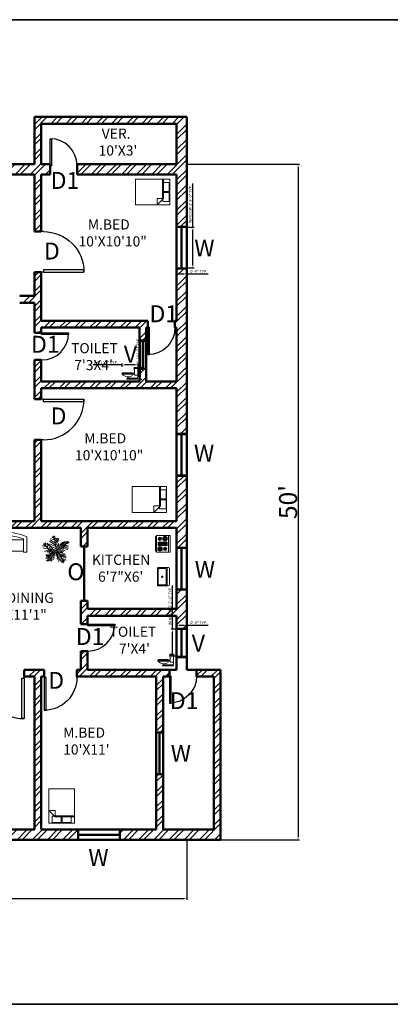
# Model space of a CAD drawing. Units: inches. Extents: x -31842 to -29388, y 18869 to 19743.
# Tile 4 of 12: x -31268 to -30939, y 18869 to 19743. Entities that reach past the tile are written whole.
import ezdxf

# ---------------------------------------------------------------- set-up
doc = ezdxf.new("R2010")
doc.units = ezdxf.units.IN
for name, color, linetype, lineweight in [('A-ANNO-DIMS', 2, 'Continuous', 18), ('A-ANNO-SYMB', 2, 'Continuous', 18), ('A-ANNO-TTLB', 7, 'Continuous', 35), ('A-AREA-IDEN', 3, 'Continuous', 18), ('A-DOOR', 3, 'Continuous', 25), ('A-FLOR-FIXT', 8, 'Continuous', 18), ('A-FURN', 8, 'Continuous', 18), ('A-GLAZ', 4, 'Continuous', 25), ('A-WALL', 7, 'Continuous', 50), ('A-WALL-PATT', 8, 'Continuous', 13), ('L-PLNT', 3, 'Continuous', 13)]:
    doc.layers.add(name, color=color, linetype=linetype, lineweight=lineweight)
doc.styles.get("Standard").update_dxf_attribs({"font": 'arial.ttf'})
doc.dimstyles.new('ISO-25', dxfattribs={"dimtxt": 2.5, "dimasz": 2.5, "dimexe": 1.25, "dimexo": 0.625, "dimtad": 1, "dimdec": 0, "dimlunit": 3, "dimtxsty": 'Standard', "dimcen": 2.5, "dimadec": 0, "dimazin": 0, "dimtfac": 1, "dimtdec": 0, "dimtmove": 0, "dimatfit": 3, "dimfxl": 1, "dimarcsym": 0})

# ---------------------------------------------------------------- blocks, each defined once
blk = doc.blocks.new('*U8')
for p, q in [((0, 0), (0, -100)), ((750, 0), (750, -100))]:
    blk.add_line(p, q)
blk.add_lwpolyline([(0, 0), (0, 750), (43.75, 750), (43.75, 0)], close=True)
blk.add_arc((0, 0), 750, 0, 90)
blk = doc.blocks.new('Bed - Queen')
for p, q in [((0, -80.00003), (0, 0)), ((0, 0), (59.99999, 0)), ((59.99999, 0), (59.99999, -80.00003)), ((0, -14.4), (44.8, -14.4)), ((44.8, -16.8), (0, -16.8)), ((7.99999, -1.2), (28.79998, -1.2)), ((7.99999, -14.4), (7.99999, -1.2)), ((28.79998, -1.2), (28.79998, -14.4)), ((31.19999, -1.2), (51.99999, -1.2)), ((31.19999, -14.4), (31.19999, -1.2)), ((59.99999, -29.6), (44.8, -14.4)), ((44.8, -14.4), (44.8, -29.6)), ((51.99999, -16.4), (46.79936, -16.4)), ((51.99999, -1.2), (51.99999, -16.4)), ((44.8, -29.6), (59.99999, -29.6)), ((59.99999, -80.00003), (0, -80.00003))]:
    blk.add_line(p, q)
blk = doc.blocks.new('Toilet - side')
for p, q in [((0.5, 5), (0.5, 22)), ((7.5, 22), (7.5, 12)), ((7.5, 21), (9, 21)), ((9, 21), (9, 20)), ((6, 8), (0.5, 8)), ((22, 2), (2, 2)), ((2, 2), (2, 1)), ((8, 10), (6, 8)), ((9, 20), (7.5, 20)), ((7.5, 12), (33, 12)), ((33, 10), (8, 10)), ((32.5, 13), (12, 13)), ((12, 13), (12, 12)), ((21, 4.5), (21, 2)), ((22, 2), (22, 4.5)), ((22, 1), (22, 2)), ((32.5, 12), (32.5, 13)), ((33, 12), (33, 10))]:
    blk.add_line(p, q)
for points in [[(0, 22), (0, 24), (8, 24), (8, 22)], [(1, 0), (1, 1), (23, 1), (23, 0)]]:
    blk.add_lwpolyline(points, close=True)
for centre, radius, start, end in [((3.8, 4.8), 3.26, 175.6013, 237.5288), ((20.3, 20.7), 16.2, 238.1872, 318.7702)]:
    blk.add_arc(centre, radius, start, end)
blk = doc.blocks.new('Range-Oven - 30 in top')
for p, q in [((0, -3), (30, -3)), ((12, -6), (18, -6)), ((13, -20), (13, -6)), ((14, -6), (14, -20)), ((15, -20), (15, -6)), ((16, -6), (16, -20)), ((17, -20), (17, -6)), ((6, -24), (6, -25)), ((8, -25), (8, -24)), ((18, -20), (12, -20)), ((22, -25), (22, -24)), ((24, -24), (24, -25))]:
    blk.add_line(p, q)
for points in [[(0, -24), (0, 0), (30, 0), (30, -24)], [(12, -21), (12, -5), (18, -5), (18, -21)], [(2, -26), (2, -25), (28, -25), (28, -26)]]:
    blk.add_lwpolyline(points, close=True)
for centre, radius in [((6, -9), 4), ((6, -9), 3), ((6, -18), 3), ((6, -9), 2), ((6, -18), 2), ((6, -9), 1), ((6, -18), 1), ((24, -18), 4), ((24, -9), 3), ((24, -18), 3), ((24, -9), 2), ((24, -18), 2), ((24, -9), 1), ((24, -18), 1)]:
    blk.add_circle(centre, radius)
blk = doc.blocks.new('Sink-single - 30 in top')
blk.add_line((-15, -3.999996), (15, -3.999996))
for points in [[(-13.5, 0), (13.5, 0)], [(-15, -18.499996), (-15, -1.5)], [(-13.5, -17.499996), (-13.5, -6.499996)], [(-12.5, -5.499996), (12.5, -5.499996)], [(13.5, -6.499996), (13.5, -17.499996)], [(15, -1.5), (15, -18.499996)], [(13.5, -19.999996), (-13.5, -19.999996)], [(12.5, -18.499996), (-12.5, -18.499996)]]:
    blk.add_lwpolyline(points)
for radius in [1, 0.5]:
    blk.add_circle((0, -11.999996), radius)
for centre, radius, start, end in [((-13.5, -1.5), 1.5, 90, 180), ((-12.5, -6.499996), 1, 90, 180), ((12.5, -6.499996), 1, 0, 90), ((13.5, -1.5), 1.5, 0, 90), ((-13.5, -18.499996), 1.5, 180, 270), ((-12.5, -17.499996), 1, 180, 270), ((12.5, -17.499996), 1, 270, 0), ((13.5, -18.499996), 1.5, 270, 0)]:
    blk.add_arc(centre, radius, start, end)
blk = doc.blocks.new('Sofa - Roundback 7 ft.')
for p, q in [((-36.000027, -34), (-36.000027, -11.4696)), ((-35.999844, -13.3819), (35.9998, -13.3819)), ((-12.00002, -32.4421), (-12.00003, -6.5971)), ((11.99997, -32.4421), (11.99998, -6.5971)), ((35.99998, -34), (35.99998, -11.4696)), ((-36.000027, -32.4421), (35.99998, -32.4421))]:
    blk.add_line(p, q)
for points in [[(-36.000027, -34), (-42.000027, -34), (-42.000027, -8)], [(41.99998, -8), (41.99998, -34), (35.99998, -34)]]:
    blk.add_lwpolyline(points)
for centre, radius, start, end in [((0, -114.25), 114.25, 68.43141, 111.5686), ((-0.00001, -127.1968), 121.1968, 72.72033, 107.2797)]:
    blk.add_arc(centre, radius, start, end)
blk = doc.blocks.new('*U122')
for p, q in [((-129.8956, 713.6638), (-626.7704, 1032.1544)), ((-185.1152, 1008.5578), (-553.1612, 1185.4942)), ((-221.9198, 1197.3052), (-433.5526, 1338.8594)), ((-258.7244, 1362.456), (-332.3336, 1421.4348)), ((0, 0), (-266.7, 1447.8)), ((-231.1146, 1315.2628), (-166.7002, 1421.4348)), ((-194.31, 1102.9442), (-65.4812, 1256.284)), ((-148.3106, 914.1968), (118.5418, 1220.9018)), ((-129.8956, 701.8528), (265.7602, 1185.4942)), ((-1206.4492, 501.3198), (-1418.082, 465.9376)), ((-1031.621, 347.98), (-1399.667, 277.1902)), ((-800.1, 114.3), (-1333.5, 647.7)), ((-847.598, 159.2326), (-1326.0578, 135.636)), ((-1234.059, 536.7274), (-1252.4486, 737.2604)), ((-718.7946, 88.4682), (-1215.644, -147.447)), ((-1105.2302, 725.4494), (-1077.6458, 395.1732)), ((-976.4268, 666.4706), (-884.4026, 194.6402)), ((-543.9664, 76.6572), (-967.2066, -206.4512)), ((-902.8176, 713.6638), (-617.5756, 100.2538)), ((0, 0), (-800.1, 114.3)), ((-369.1382, 53.086), (-783.1836, 642.874)), ((-405.9428, 53.086), (-764.794, -241.8334)), ((-93.091, 489.5342), (-700.3796, 902.3858)), ((-617.5756, 607.4918), (-74.7014, 347.98)), ((0, 0), (-571.5, -495.3)), ((-166.7002, 29.4894), (-543.9664, -206.4512)), ((-525.5514, 347.98), (-28.6766, 123.8504)), ((-74.7014, 418.7444), (219.7608, 961.39)), ((-28.6766, 171.0436), (228.9556, 678.2816)), ((0, 0), (685.8, 228.6)), ((0, 0), (457.2, -571.5)), ((100.1268, 41.275), (284.1498, 619.2774)), ((164.5412, 41.275), (661.416, -218.2368)), ((256.5654, 88.4682), (449.7832, 666.4706)), ((284.1498, 88.4682), (781.0246, -147.447)), ((412.9786, 147.447), (587.8068, 796.2392)), ((458.978, 147.447), (891.4384, -88.4682)), ((560.197, 182.8292), (698.2206, 819.8358)), ((615.4166, 194.6402), (1185.8752, 41.275)), ((685.8, 228.6), (1219.2, 914.4)), ((689.0258, 230.0224), (790.2448, 914.1968)), ((753.4148, 312.5978), (1222.6798, 159.2326)), ((808.6344, 784.4282), (827.0494, 418.7444)), ((845.439, 418.7444), (1241.0948, 277.1902)), ((891.4384, 831.6214), (946.658, 572.1096)), ((919.0482, 501.3198), (1222.6798, 454.152)), ((983.4626, 867.0036), (1066.2666, 725.4494)), ((1029.462, 654.685), (1241.0948, 631.0884)), ((1112.2914, 760.8316), (1296.3144, 784.4282)), ((1121.4862, 925.9824), (1149.0706, 831.6214)), ((-442.7474, -383.3876), (-1086.8406, -477.7486)), ((-718.7946, -737.2604), (-1086.8406, -796.2392)), ((-617.5756, -548.5384), (-1077.6458, -560.324)), ((-783.1836, -867.029), (-1077.6458, -902.4112)), ((-875.2078, -1008.5832), (-1040.8412, -1079.3476)), ((-681.9646, -666.496), (-1022.4262, -654.685)), ((-571.5, -495.3), (-952.5, -1143)), ((-829.2084, -937.7934), (-810.7934, -1126.5408)), ((-387.5278, -324.4088), (-764.794, -324.4088)), ((-737.1842, -784.4536), (-709.5744, -1114.7298)), ((-635.9652, -607.5172), (-580.771, -1150.1374)), ((-525.5514, -465.963), (-451.9422, -1126.5408)), ((-166.7002, -147.447), (-507.1618, -253.619)), ((-433.5526, -383.3876), (-323.1134, -1020.3688)), ((-341.5284, -289.0012), (-221.9198, -831.6214)), ((-240.3094, -218.2368), (-157.5054, -595.7062)), ((-120.7008, -88.4682), (-93.091, -371.5766)), ((63.3222, -76.6826), (-37.8714, -513.1308)), ((44.9326, -64.897), (615.4166, -241.8334)), ((127.7366, -159.258), (54.1274, -654.685)), ((228.9556, -289.0012), (90.932, -914.1968)), ((357.759, -430.5554), (164.5412, -1020.3688)), ((192.151, -230.0224), (817.8292, -371.5766)), ((458.978, -572.1096), (210.5406, -1161.923)), ((311.7596, -383.3876), (937.4378, -477.7486)), ((514.1976, -772.6426), (403.7838, -1138.3264)), ((412.9786, -501.3452), (919.0482, -583.9206)), ((457.2, -571.5), (685.8, -1333.5)), ((468.1982, -572.1096), (1029.462, -737.2604)), ((486.5878, -642.8994), (983.4626, -843.4324)), ((578.612, -961.39), (495.7826, -1232.7128)), ((541.8074, -831.6214), (992.6574, -1032.1544)), ((578.612, -973.1756), (873.0488, -1138.3264)), ((624.6114, -1161.923), (587.8068, -1291.6916)), ((624.6114, -1102.9442), (781.0246, -1209.1162)), ((679.8056, -1268.095), (716.6102, -1291.6916))]:
    blk.add_line(p, q)
blk = doc.blocks.new('*D197')
at = {"layer": 'A-ANNO-DIMS', "color": 0, "lineweight": -2, "transparency": 16777216}
for p, q in [((-31651.45, 19014.34), (-31651.45, 18961.52)), ((-31119.45, 19014.34), (-31119.45, 18961.52)), ((-31648.95, 18962.77), (-31121.95, 18962.77))]:
    blk.add_line(p, q, dxfattribs=at)
at = {"layer": 'A-ANNO-DIMS', "color": 0, "transparency": 16777216}
for points in [[(-31648.95, 18963.19), (-31648.95, 18962.35), (-31651.45, 18962.77)], [(-31121.95, 18963.19), (-31121.95, 18962.35), (-31119.45, 18962.77)]]:
    blk.add_solid(points, dxfattribs=at)
at = {"layer": 'Defpoints', "color": 0, "transparency": 16777216}
for p in [(-31651.45, 19014.96), (-31119.45, 19014.96), (-31119.45, 18962.77)]:
    blk.add_point(p, dxfattribs=at)
at = {"layer": 'A-ANNO-DIMS', "color": 0, "transparency": 16777216, "insert": (-31385.45, 18971.4), "char_height": 2.5, "attachment_point": 5}
blk.add_mtext('{\\H6.4x;44\'-4"}', dxfattribs=at)
blk = doc.blocks.new('*D198')
at = {"layer": 'A-ANNO-DIMS', "color": 0, "lineweight": -2, "transparency": 16777216}
for p, q in [((-31118.83, 19614.96), (-31019.53, 19614.96)), ((-31020.78, 19612.46), (-31020.78, 19017.46)), ((-31118.83, 19014.96), (-31019.53, 19014.96))]:
    blk.add_line(p, q, dxfattribs=at)
at = {"layer": 'A-ANNO-DIMS', "color": 0, "transparency": 16777216}
for points in [[(-31021.19, 19612.46), (-31020.36, 19612.46), (-31020.78, 19614.96)], [(-31021.19, 19017.46), (-31020.36, 19017.46), (-31020.78, 19014.96)]]:
    blk.add_solid(points, dxfattribs=at)
at = {"layer": 'Defpoints', "color": 0, "transparency": 16777216}
for p in [(-31119.45, 19614.96), (-31119.45, 19014.96), (-31020.78, 19014.96)]:
    blk.add_point(p, dxfattribs=at)
at = {"layer": 'A-ANNO-DIMS', "color": 0, "transparency": 16777216, "insert": (-31029.57, 19314.96), "char_height": 2.5, "attachment_point": 5, "rotation": 90}
blk.add_mtext("{\\H6.4x;50'}", dxfattribs=at)
blk = doc.blocks.new('WIN-3FT')
for p, q in [((0, 36), (9, 36)), ((4, 0), (4, 36)), ((4.5, 0), (4.5, 36)), ((5, 0), (5, 36)), ((0, 0), (9, 0))]:
    blk.add_line(p, q)
blk = doc.blocks.new('WIN-3FT-B')
for p, q in [((0, 36), (6, 36)), ((2.5, 0), (2.5, 36)), ((3, 0), (3, 36)), ((3.5, 0), (3.5, 36)), ((0, 0), (6, 0))]:
    blk.add_line(p, q)
blk = doc.blocks.new('WIN-2FT')
for p, q in [((0, 24), (9, 24)), ((4, 0), (4, 24)), ((4.5, 0), (4.5, 24)), ((5, 0), (5, 24)), ((0, 0), (9, 0))]:
    blk.add_line(p, q)
blk = doc.blocks.new('*D217')
at = {"layer": 'A-ANNO-DIMS', "color": 0, "lineweight": -2, "transparency": 16777216}
for p, q in [((-31114.05, 19558.96), (-31114.05, 19597.93)), ((-31118.83, 19558.96), (-31112.8, 19558.96)), ((-31114.05, 19525.46), (-31114.05, 19556.46)), ((-31118.83, 19522.96), (-31112.8, 19522.96))]:
    blk.add_line(p, q, dxfattribs=at)
at = {"layer": 'A-ANNO-DIMS', "color": 0, "transparency": 16777216}
for points in [[(-31114.47, 19556.46), (-31113.64, 19556.46), (-31114.05, 19558.96)], [(-31114.47, 19525.46), (-31113.64, 19525.46), (-31114.05, 19522.96)]]:
    blk.add_solid(points, dxfattribs=at)
at = {"layer": 'Defpoints', "color": 0, "transparency": 16777216}
for p in [(-31119.45, 19558.96), (-31114.05, 19558.96), (-31119.45, 19522.96)]:
    blk.add_point(p, dxfattribs=at)
at = {"layer": 'A-ANNO-DIMS', "color": 0, "transparency": 16777216, "insert": (-31115.97, 19579.69), "char_height": 2.5, "attachment_point": 5, "rotation": 90}
blk.add_mtext('WINDOW 3\' 3\'-0" TYP.', dxfattribs=at)
blk = doc.blocks.new('*D218')
at = {"layer": 'A-ANNO-DIMS', "color": 0, "lineweight": -2, "transparency": 16777216}
for p, q in [((-31128.45, 19522.34), (-31128.45, 19516.31)), ((-31119.45, 19522.34), (-31119.45, 19516.31)), ((-31125.95, 19517.56), (-31121.95, 19517.56)), ((-31119.45, 19517.56), (-31100.46, 19517.56))]:
    blk.add_line(p, q, dxfattribs=at)
at = {"layer": 'A-ANNO-DIMS', "color": 0, "transparency": 16777216}
for points in [[(-31125.95, 19517.98), (-31125.95, 19517.14), (-31128.45, 19517.56)], [(-31121.95, 19517.98), (-31121.95, 19517.14), (-31119.45, 19517.56)]]:
    blk.add_solid(points, dxfattribs=at)
at = {"layer": 'Defpoints', "color": 0, "transparency": 16777216}
for p in [(-31128.45, 19522.96), (-31119.45, 19522.96), (-31119.45, 19517.56)]:
    blk.add_point(p, dxfattribs=at)
at = {"layer": 'A-ANNO-DIMS', "color": 0, "transparency": 16777216, "insert": (-31108.71, 19519.46), "char_height": 2.5, "attachment_point": 5}
blk.add_mtext('0\'-9" TYP.', dxfattribs=at)
blk = doc.blocks.new('*D225')
at = {"layer": 'A-ANNO-DIMS', "color": 0, "lineweight": -2, "transparency": 16777216}
for p, q in [((-31176.87, 19436.68), (-31202.75, 19436.68)), ((-31176.87, 19435.17), (-31176.87, 19437.93)), ((-31165.13, 19436.68), (-31174.37, 19436.68)), ((-31162.63, 19435.17), (-31162.63, 19437.93))]:
    blk.add_line(p, q, dxfattribs=at)
at = {"layer": 'A-ANNO-DIMS', "color": 0, "transparency": 16777216}
for points in [[(-31174.37, 19437.09), (-31174.37, 19436.26), (-31176.87, 19436.68)], [(-31165.13, 19437.09), (-31165.13, 19436.26), (-31162.63, 19436.68)]]:
    blk.add_solid(points, dxfattribs=at)
at = {"layer": 'Defpoints', "color": 0, "transparency": 16777216}
for p in [(-31176.87, 19436.68), (-31176.87, 19434.54), (-31162.63, 19434.54)]:
    blk.add_point(p, dxfattribs=at)
at = {"layer": 'A-ANNO-DIMS', "color": 0, "transparency": 16777216, "insert": (-31191.06, 19438.59), "char_height": 2.5, "attachment_point": 5}
blk.add_mtext('WC 1\'-2" TYP.', dxfattribs=at)
blk = doc.blocks.new('*D226')
at = {"layer": 'A-ANNO-DIMS', "color": 0, "lineweight": -2, "transparency": 16777216}
for p, q in [((-31160.49, 19434.54), (-31160.49, 19461.3)), ((-31162.01, 19434.54), (-31159.24, 19434.54)), ((-31162.01, 19424.19), (-31159.24, 19424.19)), ((-31160.49, 19426.69), (-31160.49, 19432.04))]:
    blk.add_line(p, q, dxfattribs=at)
at = {"layer": 'A-ANNO-DIMS', "color": 0, "transparency": 16777216}
for points in [[(-31160.91, 19432.04), (-31160.08, 19432.04), (-31160.49, 19434.54)], [(-31160.91, 19426.69), (-31160.08, 19426.69), (-31160.49, 19424.19)]]:
    blk.add_solid(points, dxfattribs=at)
at = {"layer": 'Defpoints', "color": 0, "transparency": 16777216}
for p in [(-31162.63, 19434.54), (-31160.49, 19434.54), (-31162.63, 19424.19)]:
    blk.add_point(p, dxfattribs=at)
at = {"layer": 'A-ANNO-DIMS', "color": 0, "transparency": 16777216, "insert": (-31162.41, 19449.17), "char_height": 2.5, "attachment_point": 5, "rotation": 90}
blk.add_mtext('0\'-10 1/2" TYP.', dxfattribs=at)
blk = doc.blocks.new('*D259')
at = {"layer": 'A-ANNO-DIMS', "color": 0, "lineweight": -2, "transparency": 16777216}
for p, q in [((-31132.05, 19201.96), (-31132.05, 19240.93)), ((-31129.08, 19201.96), (-31133.3, 19201.96)), ((-31132.05, 19180.46), (-31132.05, 19199.46)), ((-31129.08, 19177.96), (-31133.3, 19177.96))]:
    blk.add_line(p, q, dxfattribs=at)
at = {"layer": 'A-ANNO-DIMS', "color": 0, "transparency": 16777216}
for points in [[(-31132.47, 19199.46), (-31131.64, 19199.46), (-31132.05, 19201.96)], [(-31132.47, 19180.46), (-31131.64, 19180.46), (-31132.05, 19177.96)]]:
    blk.add_solid(points, dxfattribs=at)
at = {"layer": 'Defpoints', "color": 0, "transparency": 16777216}
for p in [(-31132.05, 19201.96), (-31128.45, 19201.96), (-31128.45, 19177.96)]:
    blk.add_point(p, dxfattribs=at)
at = {"layer": 'A-ANNO-DIMS', "color": 0, "transparency": 16777216, "insert": (-31133.97, 19222.69), "char_height": 2.5, "attachment_point": 5, "rotation": 90}
blk.add_mtext('WINDOW 2\' 2\'-0" TYP.', dxfattribs=at)
blk = doc.blocks.new('*D260')
at = {"layer": 'A-ANNO-DIMS', "color": 0, "lineweight": -2, "transparency": 16777216}
for p, q in [((-31128.45, 19202.59), (-31128.45, 19206.81)), ((-31125.95, 19205.56), (-31121.95, 19205.56)), ((-31119.45, 19202.59), (-31119.45, 19206.81)), ((-31119.45, 19205.56), (-31100.46, 19205.56))]:
    blk.add_line(p, q, dxfattribs=at)
at = {"layer": 'A-ANNO-DIMS', "color": 0, "transparency": 16777216}
for points in [[(-31125.95, 19205.98), (-31125.95, 19205.14), (-31128.45, 19205.56)], [(-31121.95, 19205.98), (-31121.95, 19205.14), (-31119.45, 19205.56)]]:
    blk.add_solid(points, dxfattribs=at)
at = {"layer": 'Defpoints', "color": 0, "transparency": 16777216}
for p in [(-31119.45, 19205.56), (-31128.45, 19201.96), (-31119.45, 19201.96)]:
    blk.add_point(p, dxfattribs=at)
at = {"layer": 'A-ANNO-DIMS', "color": 0, "transparency": 16777216, "insert": (-31108.71, 19207.46), "char_height": 2.5, "attachment_point": 5}
blk.add_mtext('0\'-9" TYP.', dxfattribs=at)

msp = doc.modelspace()

# ---------------------------------------------------------------- hatches: boundary and pattern name
at = {"layer": 'A-WALL-PATT'}
h = msp.add_hatch(dxfattribs=at)
h.set_pattern_fill('ANSI32', color=256)
h.paths.add_polyline_path([(-31119.45, 19656.96), (-31254.45, 19656.96), (-31254.45, 19614.96), (-31277.45, 19614.96), (-31277.45, 19605.96), (-31254.45, 19605.96), (-31254.45, 19555.2), (-31248.45, 19555.2), (-31248.45, 19605.96), (-31240.75, 19605.96), (-31240.75, 19614.96), (-31248.45, 19614.96), (-31248.45, 19650.96), (-31128.45, 19650.96), (-31128.45, 19614.96), (-31216.75, 19614.96), (-31216.75, 19605.96), (-31128.45, 19605.96), (-31128.45, 19559.96), (-31119.45, 19559.96)])
h.paths.add_polyline_path([(-31153.94, 19473.06), (-31153.92, 19475.96), (-31248.45, 19475.96), (-31248.45, 19519.2), (-31251.45, 19519.2), (-31254.45, 19519.2), (-31254.45, 19497.96), (-31267.62, 19497.96), (-31267.62, 19491.96), (-31254.45, 19491.96), (-31254.45, 19465.12), (-31248.45, 19465.12), (-31248.45, 19469.96), (-31161.45, 19469.96), (-31161.45, 19458.96), (-31155.45, 19458.96), (-31155.45, 19469.96), (-31153.94, 19469.96)])
h.paths.add_polyline_path([(-31119.45, 19521.96), (-31128.45, 19521.96), (-31128.45, 19475.96), (-31129.92, 19475.96), (-31129.92, 19469.96), (-31128.45, 19469.96), (-31128.45, 19421.96), (-31155.45, 19421.96), (-31155.45, 19432.96), (-31161.45, 19432.96), (-31161.45, 19421.96), (-31248.45, 19421.96), (-31248.45, 19441.12), (-31254.45, 19441.12), (-31254.45, 19406.17), (-31248.45, 19406.17), (-31248.45, 19415.96), (-31128.45, 19415.96), (-31128.45, 19375.96), (-31119.45, 19375.96)])
h.paths.add_polyline_path([(-31315.45, 19614.96), (-31366.45, 19614.96), (-31366.45, 19605.96), (-31344.45, 19605.96), (-31344.45, 19456.39), (-31338.45, 19456.39), (-31338.45, 19491.96), (-31328.43, 19491.96), (-31328.43, 19497.96), (-31338.45, 19497.96), (-31338.45, 19605.96), (-31315.45, 19605.96)])
h.paths.add_polyline_path([(-31404.45, 19614.96), (-31455.1, 19614.96), (-31455.1, 19605.96), (-31432.45, 19605.96), (-31432.45, 19497.96), (-31448.67, 19497.96), (-31448.67, 19491.96), (-31432.45, 19491.96), (-31432.45, 19456.39), (-31429.07, 19456.39), (-31426.45, 19456.39), (-31426.45, 19605.96), (-31404.45, 19605.96)])
h.paths.add_polyline_path([(-31493.1, 19614.96), (-31516.45, 19614.96), (-31516.45, 19656.96), (-31651.45, 19656.96), (-31651.45, 19559.96), (-31642.45, 19559.96), (-31642.45, 19605.96), (-31556.65, 19605.96), (-31556.65, 19614.96), (-31642.45, 19614.96), (-31642.45, 19650.96), (-31522.45, 19650.96), (-31522.45, 19614.96), (-31532.65, 19614.96), (-31532.65, 19613.66), (-31532.65, 19610.46), (-31532.65, 19605.96), (-31522.45, 19605.96), (-31522.45, 19541.95), (-31516.45, 19541.95), (-31516.45, 19605.96), (-31493.1, 19605.96)])
h.paths.add_polyline_path([(-31642.45, 19521.96), (-31651.45, 19521.96), (-31651.45, 19374.96), (-31642.45, 19374.96), (-31642.45, 19415.96), (-31522.45, 19415.96), (-31522.45, 19406.54), (-31516.45, 19406.54), (-31516.45, 19441.56), (-31522.45, 19441.56), (-31522.45, 19421.96), (-31609.45, 19421.96), (-31609.45, 19432.96), (-31615.45, 19432.96), (-31615.45, 19421.96), (-31642.45, 19421.96), (-31642.45, 19469.96), (-31641.6, 19469.96), (-31641.6, 19475.96), (-31642.45, 19475.96)])
h.paths.add_polyline_path([(-31516.45, 19491.96), (-31506.54, 19491.96), (-31506.54, 19497.96), (-31516.45, 19497.96), (-31516.45, 19505.95), (-31522.45, 19505.95), (-31522.45, 19475.96), (-31617.6, 19475.96), (-31617.6, 19469.96), (-31615.45, 19469.96), (-31615.45, 19458.96), (-31609.45, 19458.96), (-31609.45, 19469.96), (-31522.45, 19469.96), (-31522.45, 19465.56), (-31516.45, 19465.56)])
h.paths.add_polyline_path([(-31248.45, 19370.17), (-31251.45, 19370.17), (-31254.45, 19370.17), (-31254.45, 19297.96), (-31338.45, 19297.96), (-31338.45, 19420.39), (-31344.45, 19420.39), (-31344.45, 19413.96), (-31346.02, 19413.96), (-31346.02, 19407.96), (-31344.45, 19407.96), (-31344.45, 19291.96), (-31213.45, 19291.96), (-31213.45, 19275.43), (-31207.45, 19275.43), (-31207.45, 19291.96), (-31128.45, 19291.96), (-31128.45, 19274.96), (-31119.45, 19274.96), (-31119.45, 19337.96), (-31128.45, 19337.96), (-31128.45, 19297.96), (-31248.45, 19297.96)])
h.paths.add_polyline_path([(-31426.45, 19407.96), (-31424.99, 19407.96), (-31424.99, 19410.83), (-31424.95, 19413.96), (-31426.45, 19413.96), (-31426.45, 19420.39), (-31432.45, 19420.39), (-31432.45, 19295.96), (-31516.45, 19295.96), (-31516.45, 19370.54), (-31522.45, 19370.54), (-31522.45, 19295.96), (-31642.45, 19295.96), (-31642.45, 19336.96), (-31651.45, 19336.96), (-31651.45, 19272.96), (-31642.45, 19272.96), (-31642.45, 19289.96), (-31563.45, 19289.96), (-31563.45, 19270.05), (-31557.45, 19270.05), (-31557.45, 19289.96), (-31426.45, 19289.96)])
h.paths.add_polyline_path([(-31557.45, 19222.83), (-31563.45, 19222.83), (-31563.45, 19217.96), (-31642.45, 19217.96), (-31642.45, 19234.96), (-31651.45, 19234.96), (-31651.45, 19201.96), (-31642.45, 19201.96), (-31642.45, 19211.96), (-31563.45, 19211.96), (-31563.45, 19206.27), (-31562.72, 19206.27), (-31559.53, 19206.27), (-31557.45, 19206.18)])
h.paths.add_polyline_path([(-31553.97, 19163.65), (-31553.95, 19165.96), (-31557.45, 19165.96), (-31557.45, 19182.18), (-31563.45, 19182.18), (-31563.45, 19165.96), (-31639.16, 19165.96), (-31639.16, 19159.96), (-31630.45, 19159.96), (-31630.45, 19110.96), (-31624.45, 19110.96), (-31624.45, 19159.96), (-31553.97, 19159.96)])
h.paths.add_polyline_path([(-31663.16, 19165.96), (-31681.45, 19165.96), (-31681.45, 19014.96), (-31592.45, 19014.96), (-31592.45, 19023.96), (-31624.45, 19023.96), (-31624.45, 19072.96), (-31630.45, 19072.96), (-31630.45, 19023.96), (-31675.45, 19023.96), (-31675.45, 19159.96), (-31663.16, 19159.96)])
h.paths.add_polyline_path([(-31516.45, 19159.96), (-31505.99, 19159.96), (-31505.99, 19165.96), (-31524.95, 19165.96), (-31524.95, 19159.96), (-31522.45, 19159.96), (-31522.45, 19023.96), (-31554.45, 19023.96), (-31554.45, 19014.96), (-31471.45, 19014.96), (-31471.45, 19023.96), (-31516.45, 19023.96)])
h.paths.add_polyline_path([(-31337.45, 19023.96), (-31382.45, 19023.96), (-31382.45, 19159.96), (-31299.75, 19159.96), (-31299.75, 19165.96), (-31344.45, 19165.96), (-31382.45, 19165.96), (-31382.45, 19407.96), (-31382.02, 19413.96), (-31388.95, 19413.96), (-31388.95, 19407.96), (-31388.45, 19407.96), (-31388.45, 19165.96), (-31432.45, 19165.96), (-31469.99, 19165.96), (-31469.99, 19159.96), (-31432.45, 19159.96), (-31388.45, 19159.96), (-31388.45, 19023.96), (-31433.45, 19023.96), (-31433.45, 19014.96), (-31337.45, 19014.96)])
h.paths.add_polyline_path([(-31216.45, 19023.96), (-31248.45, 19023.96), (-31248.45, 19159.96), (-31245.93, 19159.96), (-31245.93, 19162.87), (-31245.93, 19165.96), (-31254.45, 19165.96), (-31263.75, 19165.96), (-31263.75, 19159.96), (-31254.45, 19159.96), (-31254.45, 19023.96), (-31299.45, 19023.96), (-31299.45, 19014.96), (-31216.45, 19014.96)])
h.paths.add_polyline_path([(-31089.45, 19165.96), (-31110.75, 19165.96), (-31110.75, 19159.96), (-31095.45, 19159.96), (-31095.45, 19023.96), (-31140.45, 19023.96), (-31140.45, 19072.96), (-31146.45, 19072.96), (-31146.45, 19023.96), (-31178.45, 19023.96), (-31178.45, 19014.96), (-31089.45, 19014.96)])
h.paths.add_polyline_path([(-31134.75, 19165.96), (-31207.45, 19165.96), (-31207.45, 19182.5), (-31213.45, 19182.5), (-31213.45, 19165.96), (-31216.93, 19165.96), (-31216.93, 19159.96), (-31146.45, 19159.96), (-31146.45, 19110.96), (-31140.45, 19110.96), (-31140.45, 19159.96), (-31134.75, 19159.96)])
h.paths.add_polyline_path([(-31119.45, 19236.96), (-31128.45, 19236.96), (-31128.45, 19219.96), (-31207.45, 19219.96), (-31207.45, 19227.12), (-31213.45, 19227.12), (-31213.45, 19206.5), (-31207.45, 19206.5), (-31207.45, 19213.96), (-31128.45, 19213.96), (-31128.45, 19202.96), (-31119.45, 19202.96)])

# ---------------------------------------------------------------- linework, layer by layer
at = {"layer": 'A-ANNO-TTLB'}
msp.add_lwpolyline([(-31842.18, 19743.36), (-29387.67, 19743.36), (-29387.67, 18868.82), (-31842.18, 18868.82)], close=True, dxfattribs=at)
at = {"layer": 'A-GLAZ'}
for p, q in [((-31128.45, 19559.96), (-31119.45, 19559.96)), ((-31128.45, 19521.96), (-31119.45, 19521.96)), ((-31161.45, 19458.96), (-31155.45, 19458.96)), ((-31161.45, 19458.96), (-31155.45, 19458.96)), ((-31161.45, 19457.96), (-31155.45, 19457.96)), ((-31161.45, 19457.96), (-31155.45, 19457.96)), ((-31158.95, 19457.96), (-31158.95, 19433.96)), ((-31158.95, 19457.96), (-31158.95, 19433.96)), ((-31158.45, 19457.96), (-31158.45, 19433.96)), ((-31158.45, 19457.96), (-31158.45, 19433.96)), ((-31157.95, 19457.96), (-31157.95, 19433.96)), ((-31157.95, 19457.96), (-31157.95, 19433.96)), ((-31161.45, 19433.96), (-31155.45, 19433.96)), ((-31161.45, 19433.96), (-31155.45, 19433.96)), ((-31161.45, 19432.96), (-31155.45, 19432.96)), ((-31161.45, 19432.96), (-31155.45, 19432.96)), ((-31128.45, 19375.96), (-31119.45, 19375.96)), ((-31128.45, 19337.96), (-31119.45, 19337.96)), ((-31128.45, 19274.96), (-31119.45, 19274.96)), ((-31128.45, 19236.96), (-31119.45, 19236.96)), ((-31128.45, 19202.96), (-31119.45, 19202.96)), ((-31128.45, 19176.96), (-31119.45, 19176.96)), ((-31146.45, 19110.96), (-31140.45, 19110.96)), ((-31146.45, 19072.96), (-31140.45, 19072.96)), ((-31216.45, 19023.96), (-31216.45, 19014.96)), ((-31178.45, 19023.96), (-31178.45, 19014.96))]:
    msp.add_line(p, q, dxfattribs=at)
at = {"layer": 'A-WALL'}
for p, q in [((-31254.45, 19656.96), (-31254.45, 19614.96)), ((-31254.45, 19656.96), (-31119.45, 19656.96)), ((-31248.45, 19650.96), (-31248.45, 19614.96)), ((-31248.45, 19650.96), (-31128.45, 19650.96)), ((-31128.45, 19650.96), (-31128.45, 19614.96)), ((-31119.45, 19656.96), (-31119.45, 19165.96)), ((-31516.45, 19614.96), (-31254.45, 19614.96)), ((-31248.45, 19614.96), (-31240.75, 19614.96)), ((-31240.75, 19614.96), (-31240.75, 19605.96)), ((-31216.75, 19614.96), (-31216.75, 19605.96)), ((-31216.75, 19614.96), (-31128.45, 19614.96)), ((-31338.45, 19605.96), (-31254.45, 19605.96)), ((-31254.45, 19605.96), (-31254.45, 19555.2)), ((-31248.45, 19605.96), (-31240.75, 19605.96)), ((-31248.45, 19605.96), (-31248.45, 19555.2)), ((-31216.75, 19605.96), (-31128.45, 19605.96)), ((-31128.45, 19605.96), (-31128.45, 19475.96)), ((-31254.45, 19555.2), (-31248.45, 19555.2)), ((-31254.45, 19519.2), (-31248.45, 19519.2)), ((-31254.45, 19519.2), (-31254.45, 19497.96)), ((-31248.45, 19519.2), (-31248.45, 19475.96)), ((-31267.62, 19497.96), (-31254.45, 19497.96)), ((-31267.62, 19491.96), (-31254.45, 19491.96)), ((-31254.45, 19491.96), (-31254.45, 19465.12)), ((-31248.45, 19475.96), (-31153.92, 19475.96)), ((-31153.92, 19475.96), (-31153.92, 19469.96)), ((-31129.92, 19475.96), (-31129.92, 19469.96)), ((-31129.92, 19475.96), (-31128.45, 19475.96)), ((-31248.45, 19469.96), (-31161.45, 19469.96)), ((-31248.45, 19469.96), (-31248.45, 19465.12)), ((-31161.45, 19469.96), (-31161.45, 19421.96)), ((-31155.45, 19469.96), (-31153.92, 19469.96)), ((-31155.45, 19469.96), (-31155.45, 19421.96)), ((-31129.92, 19469.96), (-31128.45, 19469.96)), ((-31128.45, 19469.96), (-31128.45, 19421.96)), ((-31254.45, 19465.12), (-31248.45, 19465.12)), ((-31254.45, 19441.12), (-31248.45, 19441.12)), ((-31254.45, 19441.12), (-31254.45, 19406.17)), ((-31248.45, 19441.12), (-31248.45, 19421.96)), ((-31248.45, 19421.96), (-31161.45, 19421.96)), ((-31248.45, 19415.96), (-31128.45, 19415.96)), ((-31248.45, 19415.96), (-31248.45, 19406.17)), ((-31155.45, 19421.96), (-31128.45, 19421.96)), ((-31128.45, 19415.96), (-31128.45, 19297.96)), ((-31254.45, 19406.17), (-31248.45, 19406.17)), ((-31254.45, 19370.17), (-31248.45, 19370.17)), ((-31254.45, 19370.17), (-31254.45, 19297.96)), ((-31248.45, 19370.17), (-31248.45, 19297.96)), ((-31338.45, 19297.96), (-31254.45, 19297.96)), ((-31248.45, 19297.96), (-31128.45, 19297.96)), ((-31344.45, 19291.96), (-31213.45, 19291.96)), ((-31213.45, 19291.96), (-31213.45, 19275.43)), ((-31207.45, 19291.96), (-31207.45, 19275.43)), ((-31207.45, 19291.96), (-31128.45, 19291.96)), ((-31128.45, 19291.96), (-31128.45, 19219.96)), ((-31213.45, 19275.43), (-31207.45, 19275.43)), ((-31210.45, 19227.12), (-31210.45, 19275.43)), ((-31213.45, 19227.12), (-31207.45, 19227.12)), ((-31213.45, 19227.12), (-31213.45, 19206.5)), ((-31207.45, 19227.12), (-31207.45, 19219.96)), ((-31207.45, 19219.96), (-31128.45, 19219.96)), ((-31207.45, 19213.96), (-31128.45, 19213.96)), ((-31207.45, 19213.96), (-31207.45, 19206.5)), ((-31128.45, 19213.96), (-31128.45, 19165.96)), ((-31213.45, 19206.5), (-31207.45, 19206.5)), ((-31213.45, 19182.5), (-31207.45, 19182.5)), ((-31213.45, 19182.5), (-31213.45, 19165.96)), ((-31207.45, 19182.5), (-31207.45, 19165.96)), ((-31263.75, 19159.96), (-31263.75, 19165.96)), ((-31263.75, 19165.96), (-31254.45, 19165.96)), ((-31254.45, 19165.96), (-31245.93, 19165.96)), ((-31245.93, 19159.96), (-31245.93, 19165.96)), ((-31216.93, 19159.96), (-31216.93, 19165.96)), ((-31216.93, 19165.96), (-31213.45, 19165.96)), ((-31207.45, 19165.96), (-31128.45, 19165.96)), ((-31134.75, 19165.96), (-31134.75, 19159.96)), ((-31119.45, 19165.96), (-31089.45, 19165.96)), ((-31110.75, 19165.96), (-31110.75, 19159.96)), ((-31089.45, 19165.96), (-31089.45, 19014.96)), ((-31263.75, 19159.96), (-31254.45, 19159.96)), ((-31254.45, 19159.96), (-31254.45, 19023.96)), ((-31248.45, 19159.96), (-31248.45, 19023.96)), ((-31248.45, 19159.96), (-31245.93, 19159.96)), ((-31216.93, 19159.96), (-31146.45, 19159.96)), ((-31146.45, 19159.96), (-31146.45, 19023.96)), ((-31140.45, 19159.96), (-31140.45, 19023.96)), ((-31140.45, 19159.96), (-31134.75, 19159.96)), ((-31110.75, 19159.96), (-31095.45, 19159.96)), ((-31095.45, 19159.96), (-31095.45, 19023.96)), ((-31254.45, 19023.96), (-31382.45, 19023.96)), ((-31146.45, 19023.96), (-31248.45, 19023.96)), ((-31095.45, 19023.96), (-31140.45, 19023.96)), ((-31089.45, 19014.96), (-31681.45, 19014.96))]:
    msp.add_line(p, q, dxfattribs=at)

# ---------------------------------------------------------------- block references
at = {"layer": 'A-DOOR', "xscale": 0.0320000000000009, "yscale": 0.0320000000000009, "zscale": 0.0320000000000009}
msp.add_blockref('*U8', (-31240.75, 19613.66), dxfattribs=at)
at = {"layer": 'A-DOOR'}
for p, xscale, yscale, zscale, rotation in [((-31246.65, 19519.2), -0.0480000009996888, 0.0480000009996888, 0.0480000009996888, 270), ((-31153.94, 19469.86), -0.03199974142424, 0.03199974142424, 0.03199974142424, 180), ((-31248.25, 19465.12), 0.0320000009996884, 0.0320000009996884, 0.0320000009996884, 270), ((-31246.65, 19406.17), 0.0479999979369979, 0.0479999979369979, 0.0479999979369979, 270), ((-31207.25, 19206.5), 0.0320000009996884, 0.0320000009996884, 0.0320000009996884, 270), ((-31263.75, 19158.56), 0.0480000000000001, 0.0480000000000001, 0.0480000000000001, 180), ((-31245.93, 19159), -0.0386670485405529, 0.0386670485405529, 0.0386670485405529, 180), ((-31134.76, 19160.28), -0.03199974142424, 0.03199974142424, 0.03199974142424, 180)]:
    msp.add_blockref('*U8', p, dxfattribs=dict(at, xscale=xscale, yscale=yscale, zscale=zscale, rotation=rotation))
at = {"layer": 'A-FLOR-FIXT', "xscale": -0.4314503559530352, "yscale": 0.4314503559530352, "zscale": 0.4314503559530352}
for p in [(-31162.63, 19424.19), (-31130.91, 19169.34)]:
    msp.add_blockref('Toilet - side', p, dxfattribs=at)
at = {"layer": 'A-FLOR-FIXT', "rotation": 270}
for name, p, xscale, yscale, zscale in [('Range-Oven - 30 in top', (-31134.22, 19285.35), 0.501109879279097, 0.501109879279097, 0.501109879279097), ('Sink-single - 30 in top', (-31134.75, 19248.59), 0.537483841617589, 0.537483841617589, 0.537483841617589)]:
    msp.add_blockref(name, p, dxfattribs=dict(at, xscale=xscale, yscale=yscale, zscale=zscale))
at = {"layer": 'A-FURN', "xscale": 0.382279819255463, "yscale": 0.382279819255463, "zscale": 0.382279819255463}
for p, rotation in [((-31134.48, 19601.79), 270), ((-31137.36, 19328.69), 270), ((-31218.92, 19029.74), 180)]:
    msp.add_blockref('Bed - Queen', p, dxfattribs=dict(at, rotation=rotation))
at = {"layer": 'A-FURN', "xscale": 0.5237896943857897, "yscale": 0.5237896943857897, "zscale": 0.5237896943857897}
msp.add_blockref('Sofa - Roundback 7 ft.', (-31283.23, 19288.36), dxfattribs=at)
at = {"layer": 'A-GLAZ'}
for name, p in [('WIN-3FT', (-31128.45, 19522.96)), ('WIN-3FT', (-31128.45, 19338.96)), ('WIN-3FT', (-31128.45, 19237.96)), ('WIN-2FT', (-31128.45, 19177.96)), ('WIN-3FT-B', (-31146.45, 19073.96))]:
    msp.add_blockref(name, p, dxfattribs=at)
at = {"layer": 'A-GLAZ', "rotation": 269.9999999999755}
msp.add_blockref('WIN-3FT', (-31215.45, 19023.96), dxfattribs=at)
at = {"layer": 'L-PLNT', "xscale": 0.0086524126017149, "yscale": 0.0086524126017149, "zscale": 0.0086524126017149}
msp.add_blockref('*U122', (-31235.11, 19272.31), dxfattribs=at)

# ---------------------------------------------------------------- texts
at = {"layer": 'A-ANNO-SYMB', "char_height": 15, "attachment_point": 1}
for s, insert in [('{D1}', (-31240.18, 19608.06)), ('{W}', (-31112.75, 19548.1)), ('{D}', (-31246.13, 19545.35)), ('{D1}', (-31152.53, 19489.66)), ('{D1}', (-31257.61, 19462.57)), ('{V}', (-31175.29, 19453.84)), ('{D}', (-31240.21, 19398.92)), ('{W}', (-31113.09, 19365.87)), ('{O}', (-31225.4, 19260.5)), ('{W}', (-31112.36, 19262.63)), ('{D1}', (-31217.89, 19203)), ('{V}', (-31115.02, 19197.01)), ('{D}', (-31242.32, 19164.05)), ('{D1}', (-31134.52, 19145.99)), ('{W}', (-31133.66, 19099.28)), ('{W}', (-31206.75, 19006.63))]:
    msp.add_mtext_dynamic_manual_height_columns(s, width=533.5224, gutter_width=12.5, heights=[0], dxfattribs=dict(at, insert=insert))
at = {"layer": 'A-AREA-IDEN', "char_height": 2.5, "attachment_point": 1}
for s, insert in [("{\\H3.6x;    VER.\\P   10'X3'}", (-31205.87, 19646.67)), ('{\\H3.6x;   M.BED\\P10\'X10\'10"}', (-31215.43, 19565.96)), ("{\\H3.6x;  TOILET\\P   7'3X4'}", (-31227.52, 19456.09)), ('{\\H3.6x;   M.BED\\P10\'X10\'10"}', (-31218.59, 19376)), ('{\\H3.6x;KITCHEN\\P  6\'7"X6\'}', (-31203.62, 19268.15)), ('{\\H3.6x;LIVING/DINING\\P  16\'10"X11\'1"}', (-31322.33, 19234.33)), ("{\\H3.6x;TOILET\\P   7'X4'}", (-31187.84, 19204.26)), ("{\\H3.6x;M.BED\\P10'X11'}", (-31229.05, 19114.64))]:
    msp.add_mtext_dynamic_manual_height_columns(s, width=652.6959, gutter_width=12.5, heights=[0], dxfattribs=dict(at, insert=insert))

# ---------------------------------------------------------------- dimensions: what is measured, and where the dimension line sits
at = {"layer": 'A-ANNO-DIMS'}
for base, p1, p2, angle, text, override, picture, middle in [((-31020.78, 19014.96), (-31119.45, 19614.96), (-31119.45, 19014.96), 90, '{\\H6.4x;<>}', {"dimclrd": 0, "dimclre": 0, "dimclrt": 0}, '*D198', (-31029.57, 19314.96)), ((-31114.05, 19558.96), (-31119.45, 19522.96), (-31119.45, 19558.96), 90, "WINDOW 3' <> TYP.", {"dimdec": 1, "dimlfac": 1, "dimrnd": 0, "dimzin": 1, "dimdsep": 46, "dimlunit": 4, "dimfrac": 2}, '*D217', (-31115.97, 19579.69)), ((-31160.4943, 19434.5406), (-31162.63, 19424.1857), (-31162.63, 19434.5406), 90, '<> TYP.', {"dimdec": 1, "dimlfac": 1, "dimrnd": 0, "dimzin": 1, "dimdsep": 46, "dimlunit": 4, "dimfrac": 2}, '*D226', (-31162.412, 19449.1688)), ((-31176.87, 19436.68), (-31162.63, 19434.54), (-31176.87, 19434.54), 180, 'WC <> TYP.', {"dimdec": 1, "dimlfac": 1, "dimrnd": 0, "dimzin": 1, "dimdsep": 46, "dimlunit": 4, "dimfrac": 2}, '*D225', (-31191.06, 19438.59)), ((-31132.05, 19201.96), (-31128.45, 19177.96), (-31128.45, 19201.96), 90, "WINDOW 2' <> TYP.", {"dimdec": 1, "dimlfac": 1, "dimrnd": 0, "dimzin": 1, "dimdsep": 46, "dimlunit": 4, "dimfrac": 2}, '*D259', (-31133.97, 19222.69))]:
    dim = msp.add_linear_dim(base=base, p1=p1, p2=p2, angle=angle, text=text, dimstyle='ISO-25', override=override, dxfattribs=at)
    dim.commit()
    dim.dimension.update_dxf_attribs({"geometry": picture, "text_midpoint": middle})
for base, p1, p2, text, override, picture, middle in [((-31119.45, 19517.56), (-31128.45, 19522.96), (-31119.45, 19522.96), '<> TYP.', {"dimdec": 1, "dimlfac": 1, "dimrnd": 0, "dimzin": 1, "dimdsep": 46, "dimlunit": 4, "dimfrac": 2}, '*D218', (-31108.71, 19519.46)), ((-31119.45, 19205.56), (-31128.45, 19201.96), (-31119.45, 19201.96), '<> TYP.', {"dimdec": 1, "dimlfac": 1, "dimrnd": 0, "dimzin": 1, "dimdsep": 46, "dimlunit": 4, "dimfrac": 2}, '*D260', (-31108.71, 19207.46)), ((-31119.45, 18962.77), (-31651.45, 19014.96), (-31119.45, 19014.96), '{\\H6.4x;<>}', {"dimclrd": 0, "dimclre": 0, "dimclrt": 0}, '*D197', (-31385.45, 18971.4))]:
    dim = msp.add_linear_dim(base=base, p1=p1, p2=p2, text=text, dimstyle='ISO-25', override=override, dxfattribs=at)
    dim.commit()
    dim.dimension.update_dxf_attribs({"geometry": picture, "text_midpoint": middle})

doc.saveas('drawing.dxf')
